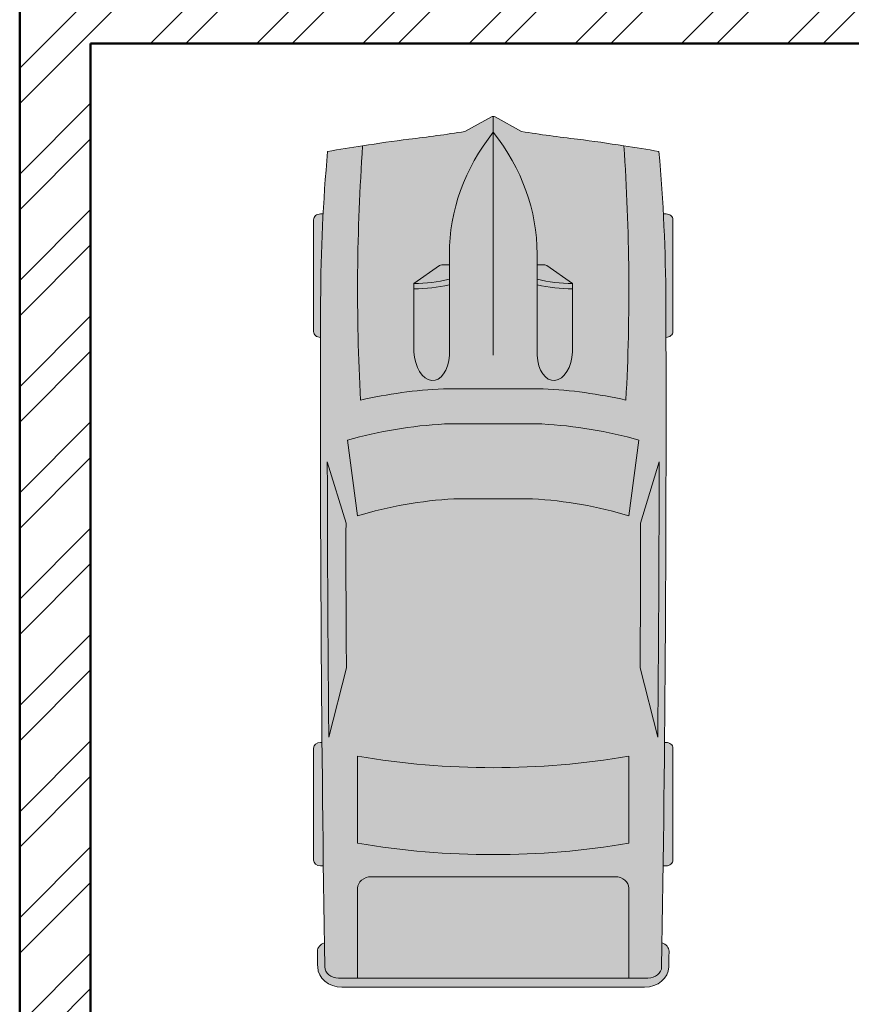
# Model space of a CAD drawing. Units: inches. Extents: x -31485 to -28799, y 18003 to 19130.
# Tile 1 of 15: x -31210 to -31104, y 18273 to 18398. Entities that reach past the tile are written whole.
import ezdxf

# ---------------------------------------------------------------- set-up
doc = ezdxf.new("R2010")
doc.units = ezdxf.units.IN
for name, color, linetype, lineweight in [('A-EQPM', 8, 'Continuous', 18), ('A-WALL', 7, 'Continuous', 50), ('A-WALL-PATT', 8, 'Continuous', 13)]:
    doc.layers.add(name, color=color, linetype=linetype, lineweight=lineweight)

# ---------------------------------------------------------------- blocks, each defined once
blk = doc.blocks.new('*U75')
for p, q in [((1182.463644577746, 987.7673041878503), (567.7039087844591, 987.7673041878503)), ((3472.124202183229, 987.7673041878503), (4086.88393797651, 987.767304187848)), ((536.0433148737552, 950.1792138851854), (536.0433148737552, 935.5404748014407)), ((1214.124238488447, 949.7089586534819), (1214.124238488447, 950.1792138851854)), ((3440.463608272525, 941.6679440245914), (3440.463608272525, 950.1792138851854)), ((4118.544531887212, 950.1792138851804), (4118.544531887212, 934.0601128753084)), ((2234.827175480885, 809.5287016048088), (1898.878785383111, 912.4126225124705)), ((3411.559256322833, 904.3494681924599), (3029.921878250559, 807.1504809911063)), ((4736.411271353851, -850.8646766016326), (4736.411271353883, 850.864676601626)), ((4785.334832293326, -832.0706314503777), (4785.334832293357, 832.0706314502926)), ((1778.76917512805, 801.0177247054045), (2194.716249451875, 745.5217224176465)), ((3515.941238262737, 745.5217224176508), (3994.062813016633, 745.5217224176508)), ((4736.411271353883, 745.5217224176529), (4242.012185201922, 745.5217224176529)), ((4178.690997380514, 670.345541812321), (4178.690997380509, -670.3455418123318)), ((819.5542361210883, 295.2827619512633), (917.6699264680983, 436.1082195367583)), ((917.6699264680983, 436.1082195367583), (1293.848362214069, 436.1082195367583)), ((815.9220749762081, 241.4481679439487), (815.9220749762081, 283.3039660446585)), ((1496.485716216861, -273.6820371142997), (1496.485716216861, 273.6820371142868)), ((756.2288711996046, 241.4481679439487), (1312.764151599097, 241.4481679439487)), ((1690.372337881975, -267.4332505757059), (1690.372337881975, 267.4332505756928)), ((4736.411271353883, -267.4332505757059), (4736.411271353883, 267.4332505756928)), ((2101.521373270556, 215.7994139342878), (2101.521373270556, -215.7994139342835)), ((82.96813941916749, 155.6585683733955), (2.596917328392246, 10.3141998552517)), ((-1.1252e-12, -6.4972e-12), (1312.764151599097, -6.4972e-12)), ((2.596917328392246, -10.31419985525964), (82.96813941916749, -155.6585683734063)), ((756.2288711996046, -241.4481679439617), (1312.764151599097, -241.4481679439617)), ((815.9220749762081, -241.4481679439617), (815.9220749762081, -283.3039660446715)), ((819.5542361210883, -295.2827619512763), (917.6699264680983, -436.1082195367712)), ((917.6699264680983, -436.1082195367712), (1293.848362214069, -436.1082195367712)), ((2194.716249451869, -745.5217224176688), (1778.769175128041, -801.0177247054262)), ((3994.062813016633, -745.5217224176616), (3515.941238262737, -745.5217224176638)), ((4242.012185201917, -745.5217224176638), (4736.411271353857, -745.5217224176594)), ((2234.827175480882, -809.5287016048153), (1898.878785383109, -912.4126225124726)), ((3411.559256322828, -904.349468192473), (3029.921878250557, -807.150480991115)), ((536.0433148737552, -950.1792138851984), (536.0433148737552, -935.5404748014537)), ((1214.124238488447, -949.7089586534948), (1214.124238488447, -950.1792138851984)), ((3440.463608272523, -941.6679440246044), (3440.463608272523, -950.1792138851984)), ((4118.544531887212, -950.1792138851933), (4118.544531887212, -934.0601128753214)), ((1182.463644577746, -987.7673041878633), (567.7039087844591, -987.7673041878633)), ((3472.124202183229, -987.7673041878633), (4086.883937976504, -987.767304187861))]:
    blk.add_line(p, q)
for centre, major_axis, ratio, start_param, end_param in [((567.7039087844591, 950.1792138851861), (5.296e-13, -37.5880903026662), 0.842303869543976, 3.141592653589776, 4.712388980384677), ((1182.463644577746, 950.1792138851861), (5.601e-13, 37.58809030266621), 0.8423038695439758, -1.570796326794884, 1.73e-14), ((3472.124202183229, 950.1792138851861), (5.988e-12, -37.5880903026662), 0.8423038695439762, 3.141592653589603, 4.712388980384554), ((4086.88393797651, 950.179213885181), (1.4197e-12, 37.5880903026662), 0.842303869543976, -1.570796326794865, 4.44e-14), ((1046.255263051279, -12467.92283887244), (3.2861e-12, 13417.14359589015), 0.8423038695439741, 0.0028100083536837, 0.0755983031096952), ((1637.842620806017, -268112.68896731), (4.8454159e-09, 269062.8681811952), 0.842303869543847, -0.0133969486112073, 0.0027970409639888), ((4587.952203166941, 910.2894362332722), (1.8792e-12, 56.38213545399769), 0.8423038695439691, -0.0130174256259048, 1.249894140392862), ((1637.84262086767, -268131.4830124673), (3.42859201765e-05, 269120.9512111412), 0.8423038681351471, -0.0133969484821159, -0.0130174254969711), ((4673.090083532475, 850.8646766015395), (7.5e-15, -75.17618060533067), 0.8423038695439952, 1.570796326796048, 3.128195704978389), ((4673.090083532448, 832.070631450172), (2.1733e-12, -133.2592106239272), 0.8423038695439737, 1.570796326795794, 3.128195704978164), ((6757.162543998887, -699.1204428451242), (4.9938223e-09, 7958.017136535005), 0.8423038695435286, 1.367075990158062, 1.391760499156098), ((1637.842620802809, -268112.6889680619), (4.87113144e-08, -269025.2800916445), 0.8423038695482963, 3.133765086725325, 3.140440689641252), ((3436.395912346701, 136.8410185571553), (5.76965e-11, 2077.023647078763), 0.8423038695439563, 1.245306111696802, 1.507880129813836), ((2433.035484508693, -93125.37499596032), (4.952654e-09, -93935.19844392464), 0.8423038695446962, 3.134048706297306, 3.14409775411291), ((6583.045501169266, -699.1204428451198), (3.826807e-09, -7754.693443154298), 0.8423038695443791, 4.528606069860317, 4.561837674556238), ((951.8333444315502, -15086.63944974413), (1.5767e-12, -15832.53653317094), 0.8423038695439826, 3.09604606856106, 3.200911180495224), ((3413.769624379244, 136.8410185571329), (1.08602e-11, -2280.347340451234), 0.84230386954398, 4.44948196380473, 4.652344057257214), ((3799.722190048092, 71.1058404433382), (2.17448e-11, -2021.323467232052), 0.842303869543983, 4.372215489277867, 4.640744122441986), ((433.884764992104, -3.6096e-12), (1.7438e-12, 3734.255266801694), 0.8423038695439766, 4.511394369635731, 4.913383591133647), ((912.0063397460013, -3.6096e-12), (1.7438e-12, 3734.255266801694), 0.8423038695439766, 4.511394369635731, 4.913383591133647), ((4242.012185201922, 670.3455418123216), (3.5405e-12, 75.17618060533239), 0.842303869543976, 5.55e-14, 1.57079632679492), ((-5194.164488957196, 1330.879982200552), (1.0466145e-09, -6374.389491984369), 0.8423038695441164, 1.385369446298923, 1.434372047871027), ((331.12799165183, 432.0470009052715), (3.125e-11, 696.3661584994836), 0.8423038695439277, 4.435146050259648, 4.718221029521873), ((360.7019022476185, 432.0470009052715), (3.125e-11, 696.3661584994836), 0.8423038695439277, 4.435146050259648, 4.718221029521873), ((1290.073045555822, 338.7781937403542), (161.0379696969085, -9.057857958340485), 0.6038335755719145, -1.39555193967809, 1.581314658479915), ((831.7523719315589, 283.3039660446593), (3.3347e-12, 18.79404515133458), 0.8423038695439091, 0.8797135699495516, 1.570796326795045), ((756.2288711996046, -1185.240851913765), (1.2998e-12, 1426.689019857713), 0.842303869543976, 7e-16, 0.5903187773915901), ((15.83029695535095, -3.6096e-12), (1.9e-15, -18.79404515133476), 0.842303869543842, 4.131459131953847, 5.293318828815531), ((756.2288711996046, 1185.240851913753), (1.01699e-11, 1426.689019857713), 0.8423038695439736, 2.55127387619821, 3.141592653589801), ((-5194.164488957196, -1330.879982200562), (1.0234792e-09, 6374.389491984348), 0.8423038695441192, -1.43437204787103, -1.385369446298926), ((3799.722190048497, -71.10584044329416), (1.038796e-10, -2021.323467232635), 0.8423038695439419, -1.499151468852248, -1.230622835688196), ((331.12799165183, -432.0470009052816), (3.1922e-11, -696.3661584994801), 0.842303869543932, 1.564964277657711, 1.848039256919935), ((360.7019022476185, -432.0470009052816), (3.1922e-11, -696.3661584994801), 0.842303869543932, 1.564964277657711, 1.848039256919935), ((3436.395912346742, -136.8410185572101), (8.13766e-11, -2077.023647078826), 0.8423038695439492, -1.50788012981387, -1.245306111696839), ((831.7523719315589, -283.3039660446737), (3.3028e-12, -18.79404515133458), 0.8423038695439093, 4.712388980384541, 5.403471737230034), ((3413.769624379237, -136.841018557156), (1.090899e-10, -2280.347340451348), 0.8423038695439354, -1.510751403667474, -1.307889310215002), ((6583.045501169163, 699.1204428449458), (2.756795e-10, 7754.693443157768), 0.8423038695439974, 1.721347632622872, 1.754579237318777), ((4242.012185201917, -670.3455418123318), (2.579e-13, -75.17618060533128), 0.8423038695439885, 4.712388980384686, 6.283185307179581), ((6757.162543998887, 699.1204428451076), (2.2231118e-09, 7958.017136528592), 0.8423038695441819, 1.749832154434603, 1.774516663432659), ((951.8333444315729, 15086.63944974408), (2.97009e-11, -15832.5365331709), 0.8423038695439528, -0.0593185269054384, 0.0455465850287298), ((2433.03548450906, 93125.37499596029), (4.1600574e-09, -93935.19844392457), 0.8423038695447548, -0.0025051005232382, 0.007543947292366), ((4673.090083532448, -850.8646766015358), (2.354e-13, 75.17618060532999), 0.8423038695439732, 3.154989602201626, 4.71238898038339), ((4673.090083532349, -832.0706314501077), (6.1679e-12, -133.2592106240062), 0.8423038695439807, 0.0133969486110846, 1.570796326792831), ((1046.255263051284, 12467.92283887242), (3.49903e-10, -13417.14359589015), 0.8423038695440652, -0.0755983031097181, -0.0028100083537155), ((1637.842620803916, 268112.6889680615), (4.0766478e-08, -269025.280091644), 0.8423038695397146, 0.0011519639481523, 0.0078275668641468), ((567.7039087844591, -950.1792138851977), (5.601e-13, 37.58809030266621), 0.8423038695439758, 1.570796326794908, 3.14159265358981), ((1637.842620801787, 268112.6889680619), (1.55395844e-08, 269062.868181947), 0.8423038695458147, 3.138795612625926, 3.154989602201039), ((1182.463644577746, -950.1792138851977), (5.296e-13, -37.5880903026662), 0.842303869543976, -1.69e-14, 1.570796326794884), ((3472.124202183229, -950.1792138851955), (3.96e-13, -37.58809030266733), 0.8423038695440105, -1.570796326794875, -1.27e-14), ((4086.883937976504, -950.1792138851933), (5.0003e-12, 37.58809030266732), 0.8423038695440109, 3.141592653589951, 4.712388980384771), ((4587.952203166856, -910.2894362333229), (5.777e-12, -56.38213545402103), 0.8423038695439803, -1.249894138785958, 0.0130174256254374), ((1637.842620726191, 268131.4830135791), (2.37878358395e-05, 269120.9512123862), 0.8423038705260315, 3.154610079306566, 3.154989602290631)]:
    blk.add_ellipse(centre, major_axis=major_axis, ratio=ratio, start_param=start_param, end_param=end_param)
at = {"extrusion": (0, 0, -1)}
blk.add_ellipse((1290.073045555822, -338.7781937403665), major_axis=(161.0379696969085, 9.057857958340424), ratio=0.6038335755719145, start_param=-1.39555193967809, end_param=1.581314658479915, dxfattribs=at)

msp = doc.modelspace()

# ---------------------------------------------------------------- hatches: boundary and pattern name
at = {"layer": 'A-EQPM'}
h = msp.add_hatch(color=256, dxfattribs=at)
h.dxf.hatch_style = 1
edge = h.paths.add_edge_path()
edge.add_ellipse((-24963.89229182593, 18347.74966155698), major_axis=(6207.481987576119, 3.1368e-12), ratio=0.84230386954367, start_angle=180.3838667787923, end_angle=180.5282714718174, ccw=False)
edge.add_line((-31171.17791802856, 18306.16184460638), (-31171.37427940205, 18306.16184460638))
edge.add_ellipse((-31171.37427940205, 18305.43141098043), major_axis=(-0.8671854094100128, 1.6795e-12), ratio=0.8423038695444475, start_angle=-89.99999999988903, end_angle=1.109639e-10)
edge.add_line((-31172.24146481146, 18305.43141098043), (-31172.24146481146, 18291.24844321379))
edge.add_ellipse((-31171.37427940205, 18291.24844321379), major_axis=(-0.8671854094100128, 3.5068e-12), ratio=0.8423038695402523, start_angle=2.317008e-10, end_angle=90.0000000002317)
edge.add_line((-31171.37427940205, 18290.51800958783), (-31171.00239966313, 18290.51800958783))
edge = h.paths.add_edge_path()
edge.add_ellipse((-31133.98755896982, 18287.66951830704), major_axis=(-1.734370818820025, 1.15572e-11), ratio=0.8423038695444475, start_angle=180.0000000003817, end_angle=270.0000000003818)
edge.add_line((-31133.98755896982, 18289.13038555896), (-31164.91830689776, 18289.13038555896))
edge.add_ellipse((-31164.91830689776, 18287.66951830704), major_axis=(1.734370818820025, 1.15576e-11), ratio=0.8423038695444475, start_angle=89.99999999961817, end_angle=179.9999999996181)
edge.add_line((-31166.65267771658, 18287.66951830704), (-31166.65267771658, 18276.26336091826))
edge.add_line((-31166.65267771658, 18276.26336091826), (-31132.253188151, 18276.26336091826))
edge.add_line((-31132.253188151, 18276.26336091826), (-31132.253188151, 18287.66951830704))
edge = h.paths.add_edge_path()
edge.add_ellipse((-31127.53158646552, 18305.43141098043), major_axis=(0.8671854094100124, 1.6795e-12), ratio=0.8423038695444477, start_angle=-1.109639e-10, end_angle=89.99999999988906)
edge.add_line((-31127.53158646552, 18306.16184460638), (-31127.72794783902, 18306.16184460638))
edge.add_ellipse((-37335.0135740243, 18347.74966155688), major_axis=(6207.481987558772, 4.152598e-10), ratio=0.8423038695472291, start_angle=-0.5282714718218244, end_angle=-0.38386677879640274, ccw=False)
edge.add_line((-31127.90346620446, 18290.51800958783), (-31127.53158646552, 18290.51800958783))
edge.add_ellipse((-31127.53158646552, 18291.24844321379), major_axis=(0.8671854094100124, 3.5068e-12), ratio=0.8423038695402528, start_angle=269.9999999997683, end_angle=359.9999999997682)
edge.add_line((-31126.66440105611, 18291.24844321379), (-31126.66440105611, 18305.43141098043))
edge = h.paths.add_edge_path()
edge.add_ellipse((-31497.51301000847, 18363.5764096146), major_axis=(365.2684817172168, 5.54988e-11), ratio=0.8423038695419378, start_angle=-2.198540565964143, end_angle=2.863714607828726)
edge.add_ellipse((-31165.58216542667, 18233.66012548605), major_axis=(-178.9065886093012, 1.2581094e-09), ratio=0.8423038695391548, start_angle=257.5553727069574, end_angle=259.7904610032577)
edge.add_ellipse((-31118.74853446752, 18505.36918505117), major_axis=(147.0619421407358, 1.9919546e-09), ratio=0.8423038695542743, start_angle=257.4450673550873, end_angle=260.74343399202326, ccw=False)
edge.add_line((-31145.86177312077, 18383.62178096662), (-31149.21497661432, 18385.47600528534))
edge.add_ellipse((-31149.45293293379, 18385.17070130109), major_axis=(-0.4335927046986816, 0), ratio=0.842303869552539, start_angle=232.0668695399768, end_angle=270)
edge.add_line((-31149.45293293379, 18385.53591811407), (-31149.45293293379, 18383.52118674771))
edge.add_ellipse((-31176.79732753163, 18368.08915138563), major_axis=(-32.91478475822442, 2.78257e-11), ratio=0.8423038695443898, start_angle=180.0000000000485, end_angle=209.438569598032, ccw=False)
edge.add_line((-31143.8825427734, 18368.08915138563), (-31143.8825427734, 18366.71198444421))
edge.add_line((-31143.8825427734, 18366.71198444421), (-31142.76081172944, 18366.71198444421))
edge.add_line((-31142.76081172944, 18366.71198444421), (-31139.39158951728, 18364.36458526691))
edge.add_line((-31139.39158951728, 18364.36458526691), (-31139.39158951728, 18355.68586687004))
edge.add_ellipse((-31141.63706614534, 18355.77296625432), major_axis=(0.2089715704820894, 3.715266632531377), ratio=0.6038335755718302, start_angle=106.3425919542722, end_angle=270.9979857249977, ccw=False)
edge.add_line((-31143.8825427734, 18355.24946543463), (-31143.8825427734, 18368.08915138563))
edge.add_ellipse((-31176.79732753163, 18368.08915138563), major_axis=(-32.91478475822442, 2.78257e-11), ratio=0.8423038695443898, start_angle=180.0000000000484, end_angle=209.4385695980319)
edge.add_ellipse((-31122.10853833595, 18368.08915138563), major_axis=(32.91478475822442, 2.78184e-11), ratio=0.8423038695443903, start_angle=150.561430401968, end_angle=179.9999999999515)
edge.add_line((-31155.02332309417, 18368.08915138563), (-31155.02332309417, 18355.24946543463))
edge.add_ellipse((-31157.26879972223, 18355.77296625432), major_axis=(-0.2089715704820894, 3.715266632531377), ratio=0.6038335755718302, start_angle=89.0020142750023, end_angle=253.6574080457279, ccw=False)
edge.add_line((-31159.51427635029, 18355.68586687004), (-31159.51427635029, 18364.36458526691))
edge.add_line((-31159.51427635029, 18364.36458526691), (-31156.14505413814, 18366.71198444421))
edge.add_line((-31156.14505413814, 18366.71198444421), (-31155.02332309417, 18366.71198444421))
edge.add_line((-31155.02332309417, 18366.71198444421), (-31155.02332309417, 18368.08915138563))
edge.add_ellipse((-31122.10853833595, 18368.08915138563), major_axis=(32.91478475822442, 2.78184e-11), ratio=0.8423038695443903, start_angle=150.5614304019681, end_angle=179.9999999999516, ccw=False)
edge.add_line((-31149.45293293379, 18383.52118674771), (-31149.45293293379, 18385.53591811407))
edge.add_ellipse((-31149.45293293379, 18385.17070130109), major_axis=(-0.4335927046986816, 0), ratio=0.842303869552539, start_angle=270, end_angle=307.9331304600232)
edge.add_line((-31149.69088925326, 18385.47600528534), (-31153.0440927468, 18383.62178096662))
edge.add_ellipse((-31180.15733140006, 18505.36918505117), major_axis=(-147.0619421372835, 4.9907306e-09), ratio=0.8423038695736066, start_angle=99.2565660091451, end_angle=102.55493264608151, ccw=False)
edge.add_ellipse((-31133.32370044092, 18233.66012548605), major_axis=(178.9065886092977, 1.2789651e-09), ratio=0.8423038695391513, start_angle=100.209538996733, end_angle=102.4446272930335)
edge.add_ellipse((-30801.39285585912, 18363.5764096146), major_axis=(365.2684817172171, 7.18011e-11), ratio=0.8423038695434502, start_angle=177.1362853921513, end_angle=182.1985405659441)
edge.add_ellipse((-31152.60995777187, 18306.77769481758), major_axis=(52.60932189168197, 7.16232e-11), ratio=0.8423038695431074, start_angle=94.08241069107589, end_angle=107.71995322267611, ccw=False)
edge.add_line((-31155.76698260995, 18351.01087126963), (-31143.13888325764, 18351.01087126963))
edge.add_ellipse((-31146.29590809571, 18306.77769481758), major_axis=(-52.6093218916263, 2.96862e-11), ratio=0.842303869543985, start_angle=252.2800467772827, end_angle=265.9175893088832, ccw=False)
h = msp.add_hatch(color=256, dxfattribs=at)
h.dxf.hatch_style = 1
edge = h.paths.add_edge_path()
edge.add_ellipse((-37335.0135740243, 18347.74966155688), major_axis=(6207.481987558772, 4.152598e-10), ratio=0.8423038695472291, start_angle=-0.3838667787963561, end_angle=0.0902290885904628)
edge.add_ellipse((-37335.0135740243, 18347.74966155688), major_axis=(6207.481987558772, 4.152598e-10), ratio=0.8423038695472291, start_angle=0.0902290885904628, end_angle=0.1349865768543979)
edge.add_ellipse((-31437.09725549581, 18361.39802519826), major_axis=(309.5435567121417, 3.12922e-11), ratio=0.8423038695440732, start_angle=0.1356123904321818, end_angle=2.179950313639523)
edge.add_ellipse((-31437.09725549581, 18361.39802519826), major_axis=(309.5435567121417, 3.12922e-11), ratio=0.8423038695440732, start_angle=2.179950313639523, end_angle=3.650427585692763)
edge.add_ellipse((-31165.58216542667, 18229.64311483572), major_axis=(183.5974185536168, 2.07254122e-08), ratio=0.8423038696260594, start_angle=76.2194710040335, end_angle=77.87403444124779)
edge.add_ellipse((-31497.51301000847, 18363.5764096146), major_axis=(365.2684817172168, 5.54988e-11), ratio=0.8423038695419378, start_angle=-2.1985405659640946, end_angle=2.8637146078286833, ccw=False)
edge.add_ellipse((-31146.29590809571, 18306.77769481758), major_axis=(-52.6093218916263, 2.96862e-11), ratio=0.842303869543985, start_angle=252.2800467772827, end_angle=265.9175893088831)
edge.add_line((-31143.13888325764, 18351.01087126963), (-31155.76698260995, 18351.01087126963))
edge.add_ellipse((-31152.60995777187, 18306.77769481758), major_axis=(52.60932189168197, 7.16232e-11), ratio=0.8423038695431074, start_angle=94.08241069107586, end_angle=107.719953222676)
edge.add_ellipse((-30801.39285585912, 18363.5764096146), major_axis=(365.2684817172171, 7.18011e-11), ratio=0.8423038695434502, start_angle=177.1362853921513, end_angle=182.1985405659441, ccw=False)
edge.add_ellipse((-31133.32370044092, 18229.64311483572), major_axis=(-183.5974185535601, 2.07797544e-08), ratio=0.8423038696263095, start_angle=-77.87403444123211, end_angle=-76.21947100401783)
edge.add_ellipse((-30861.80861037177, 18361.39802519826), major_axis=(-309.5435567121417, 3.20483e-11), ratio=0.8423038695440663, start_angle=-3.650427585692615, end_angle=-2.179950313639383)
edge.add_ellipse((-30861.80861037177, 18361.39802519826), major_axis=(-309.5435567121417, 3.20483e-11), ratio=0.8423038695440663, start_angle=-2.179950313639383, end_angle=-0.1356123904320413)
edge.add_ellipse((-24963.89229182593, 18347.74966155698), major_axis=(6207.481987576119, 3.1368e-12), ratio=0.84230386954367, start_angle=179.8650134231429, end_angle=179.9097709114068)
edge.add_ellipse((-24963.89229182593, 18347.74966155698), major_axis=(6207.481987576119, 3.1368e-12), ratio=0.84230386954367, start_angle=179.9097709114068, end_angle=180.3838667787923)
edge.add_ellipse((-24963.89229182593, 18347.74966155698), major_axis=(6207.481987576119, 3.1368e-12), ratio=0.84230386954367, start_angle=180.3838667787923, end_angle=180.5282714718173)
edge.add_ellipse((-24963.89229182593, 18347.74966155698), major_axis=(6207.481987576119, 3.1368e-12), ratio=0.84230386954367, start_angle=180.5282714718173, end_angle=180.6465540970609)
edge.add_ellipse((-31169.08301860692, 18277.72422817018), major_axis=(1.734370818820398, 6.2835e-12), ratio=0.8423038695442665, start_angle=180.6465540968934, end_angle=269.9999999996497)
edge.add_line((-31169.08301860692, 18276.26336091826), (-31166.65267771658, 18276.26336091826))
edge.add_line((-31166.65267771658, 18276.26336091826), (-31166.65267771658, 18287.86198447103))
edge.add_ellipse((-31164.91830689776, 18287.66951830704), major_axis=(1.734370818820025, 1.15576e-11), ratio=0.8423038695444475, start_angle=89.99999999961818, end_angle=179.9999999996182, ccw=False)
edge.add_line((-31164.91830689776, 18289.13038555896), (-31133.75905929062, 18289.13038555896))
edge.add_ellipse((-31133.98755896982, 18287.66951830704), major_axis=(-1.734370818820025, 1.15572e-11), ratio=0.8423038695444475, start_angle=180.0000000003818, end_angle=270.00000000038176, ccw=False)
edge.add_line((-31132.253188151, 18287.66951830704), (-31132.253188151, 18276.26336091826))
edge.add_line((-31132.253188151, 18276.26336091826), (-31129.82284726066, 18276.26336091826))
edge.add_ellipse((-31129.82284726066, 18277.72422817017), major_axis=(-1.734370818820364, 1.2413e-12), ratio=0.8423038695421853, start_angle=90.00000000018369, end_angle=179.3534459030602)
edge.add_ellipse((-37335.0135740243, 18347.74966155688), major_axis=(6207.481987558772, 4.152598e-10), ratio=0.8423038695472291, start_angle=-0.6465540970657812, end_angle=-0.6186431963230548)
edge.add_ellipse((-37335.0135740243, 18347.74966155688), major_axis=(6207.481987558772, 4.152598e-10), ratio=0.8423038695472291, start_angle=-0.6186431963230548, end_angle=-0.5282714718217923)
edge.add_ellipse((-37335.0135740243, 18347.74966155688), major_axis=(6207.481987558772, 4.152598e-10), ratio=0.8423038695472291, start_angle=-0.5282714718217923, end_angle=-0.3838667787963561)
edge = h.paths.add_edge_path(flags=16)
edge.add_ellipse((-29000.98074953765, 18329.40396632424), major_axis=(2167.155417170915, 1.2045892e-09), ratio=0.8423038695205244, start_angle=179.8791026309351, end_angle=180.3640763488582)
edge.add_line((-31168.07449935754, 18315.63334995188), (-31170.31695282702, 18306.82868966495))
edge.add_ellipse((-24963.89229182594, 18347.74966155692), major_axis=(6206.614802166701, 5.2511138e-09), ratio=0.842303869515611, start_angle=180.0555943134506, end_angle=180.3777641938611, ccw=False)
edge.add_line((-31170.5029758392, 18341.72736163617), (-31168.12936668919, 18333.97678053823))
edge = h.paths.add_edge_path(flags=16)
edge.add_ellipse((-31151.09339795501, 18297.87347991926), major_axis=(46.63344704056234, 1.445442e-10), ratio=0.842303869541784, start_angle=94.8700695969603, end_angle=112.7919148774121)
edge.add_line((-31166.65267771658, 18334.9021696583), (-31167.93301207454, 18344.49838034726))
edge.add_ellipse((-31152.60995777187, 18306.25568939947), major_axis=(47.91849192778146, 1.460375e-10), ratio=0.8423038695419556, start_angle=94.27742096287608, end_angle=111.8349537965307, ccw=False)
edge.add_line((-31155.62281842206, 18346.5377616215), (-31143.28304744552, 18346.5377616215))
edge.add_ellipse((-31146.29590809571, 18306.25568939947), major_axis=(-47.91849192778267, 1.361529e-10), ratio=0.8423038695419347, start_angle=248.1650462034528, end_angle=265.72257903710704, ccw=False)
edge.add_line((-31130.97285379305, 18344.49838034726), (-31132.253188151, 18334.9021696583))
edge.add_ellipse((-31147.81246791256, 18297.87347991927), major_axis=(-46.63344704055716, 1.546607e-10), ratio=0.8423038695417213, start_angle=247.208085122601, end_angle=265.1299304030565)
edge.add_line((-31144.47427874796, 18337.05224528612), (-31154.43158711963, 18337.05224528612))
edge = h.paths.add_edge_path(flags=16)
edge.add_ellipse((-31149.45293293379, 18375.52587146003), major_axis=(-86.15206721880882, 2.44e-14), ratio=0.8423038695434939, start_angle=76.40186530976904, end_angle=103.5981346902309)
edge.add_line((-31132.253188151, 18304.42051912437), (-31132.253188151, 18293.38989612087))
edge.add_ellipse((-31149.45293293379, 18364.49524845652), major_axis=(-86.15206721880666, 5.3e-15), ratio=0.8423038695434728, start_angle=76.40186530976843, end_angle=103.59813469023157, ccw=False)
edge.add_line((-31166.65267771658, 18293.38989612087), (-31166.65267771658, 18304.42051912437))
edge = h.paths.add_edge_path(flags=16)
edge.add_ellipse((-33297.92511632993, 18329.40396632425), major_axis=(-2167.155417170915, 1.2310555e-09), ratio=0.8423038695201377, start_angle=179.6359236511422, end_angle=180.1208973690652)
edge.add_line((-31130.77649917839, 18333.97678053823), (-31128.40289002838, 18341.72736163617))
edge.add_ellipse((-37335.01357404164, 18347.74966155695), major_axis=(-6206.614802166709, 5.3834157e-09), ratio=0.8423038695157945, start_angle=179.6222358061399, end_angle=179.9444056865504, ccw=False)
edge.add_line((-31128.58891304056, 18306.82868966495), (-31130.83136651004, 18315.63334995188))
h = msp.add_hatch(color=256, dxfattribs=at)
h.dxf.hatch_style = 1
edge = h.paths.add_edge_path()
edge.add_ellipse((-31127.53158646552, 18305.43141098043), major_axis=(0.8671854094100124, 1.6795e-12), ratio=0.8423038695444477, start_angle=-1.109639e-10, end_angle=89.99999999988906)
edge.add_line((-31127.53158646552, 18306.16184460638), (-31127.72794783902, 18306.16184460638))
edge.add_ellipse((-37335.0135740243, 18347.74966155688), major_axis=(6207.481987558772, 4.152598e-10), ratio=0.8423038695472291, start_angle=-0.5282714718218244, end_angle=-0.38386677879640274, ccw=False)
edge.add_line((-31127.90346620446, 18290.51800958783), (-31127.53158646552, 18290.51800958783))
edge.add_ellipse((-31127.53158646552, 18291.24844321379), major_axis=(0.8671854094100124, 3.5068e-12), ratio=0.8423038695402528, start_angle=269.9999999997683, end_angle=359.9999999997682)
edge.add_line((-31126.66440105611, 18291.24844321379), (-31126.66440105611, 18305.43141098043))
edge = h.paths.add_edge_path()
edge.add_line((-31171.17791802856, 18306.16184460638), (-31171.37427940205, 18306.16184460638))
edge.add_ellipse((-31171.37427940205, 18305.43141098043), major_axis=(-0.8671854094100128, 1.6795e-12), ratio=0.8423038695444475, start_angle=-89.99999999988903, end_angle=1.109639e-10)
edge.add_line((-31172.24146481146, 18305.43141098043), (-31172.24146481146, 18291.24844321379))
edge.add_ellipse((-31171.37427940205, 18291.24844321379), major_axis=(-0.8671854094100128, 3.5068e-12), ratio=0.8423038695402523, start_angle=2.317008e-10, end_angle=90.0000000002317)
edge.add_line((-31171.37427940205, 18290.51800958783), (-31171.00239966313, 18290.51800958783))
edge.add_ellipse((-24963.89229182593, 18347.74966155698), major_axis=(6207.481987576119, 3.1368e-12), ratio=0.84230386954367, start_angle=180.3838667787923, end_angle=180.5282714718174, ccw=False)
edge = h.paths.add_edge_path()
edge.add_ellipse((-31127.53158646552, 18372.43856353717), major_axis=(0.8671854094100124, 1.6795e-12), ratio=0.8423038695444477, start_angle=-1.109639e-10, end_angle=89.99999999988906)
edge.add_line((-31127.53158646552, 18373.16899716313), (-31127.86931314553, 18373.16899716313))
edge.add_ellipse((-31437.09725549581, 18361.39802519826), major_axis=(309.5435567121417, 3.12922e-11), ratio=0.8423038695440732, start_angle=0.1356123904321862, end_angle=2.1799503136394947, ccw=False)
edge.add_ellipse((-37335.0135740243, 18347.74966155688), major_axis=(6207.481987558772, 4.152598e-10), ratio=0.8423038695472291, start_angle=0.09022908859049039, end_angle=0.13498657685437365, ccw=False)
edge.add_line((-31127.5424356061, 18357.52516214458), (-31127.53158646552, 18357.52516214458))
edge.add_ellipse((-31127.53158646552, 18358.25559577054), major_axis=(-0.8671854094100128, 1.6795e-12), ratio=0.8423038695444475, start_angle=90.00000000011094, end_angle=180.0000000001109)
edge.add_line((-31126.66440105611, 18358.25559577054), (-31126.66440105611, 18372.43856353717))
edge = h.paths.add_edge_path()
edge.add_ellipse((-30861.80861037177, 18361.39802519826), major_axis=(-309.5435567121417, 3.20483e-11), ratio=0.8423038695440663, start_angle=-2.179950313639381, end_angle=-0.13561239043201567, ccw=False)
edge.add_line((-31171.03655272206, 18373.16899716313), (-31171.37427940205, 18373.16899716313))
edge.add_ellipse((-31171.37427940205, 18372.43856353717), major_axis=(-0.8671854094100128, 1.6795e-12), ratio=0.8423038695444475, start_angle=-89.99999999988903, end_angle=1.109639e-10)
edge.add_line((-31172.24146481146, 18372.43856353717), (-31172.24146481146, 18358.25559577054))
edge.add_ellipse((-31171.37427940205, 18358.25559577054), major_axis=(0.8671854094100124, 1.6795e-12), ratio=0.8423038695444477, start_angle=179.999999999889, end_angle=269.999999999889)
edge.add_line((-31171.37427940205, 18357.52516214458), (-31171.36343026148, 18357.52516214458))
edge.add_ellipse((-24963.89229182593, 18347.74966155698), major_axis=(6207.481987576119, 3.1368e-12), ratio=0.84230386954367, start_angle=179.865013423143, end_angle=179.9097709114068, ccw=False)
edge = h.paths.add_edge_path()
edge.add_ellipse((-31139.48528487433, 18377.21425494213), major_axis=(16.06568908904641, 9.1463e-11), ratio=0.8423038695487669, start_angle=251.332504507076, end_angle=270.3967098596572, ccw=False)
edge.add_line((-31143.8825427734, 18364.19880697911), (-31143.8825427734, 18355.24946543463))
edge.add_ellipse((-31141.63706614534, 18355.77296625432), major_axis=(0.2089715704820894, 3.715266632531377), ratio=0.6038335755718302, start_angle=106.3425919542721, end_angle=270.9979857249977)
edge.add_line((-31139.39158951728, 18355.68586687004), (-31139.39158951728, 18363.68229298866))
edge = h.paths.add_edge_path()
edge.add_ellipse((-31142.91689814715, 18366.34676763123), major_axis=(-0.4335927047225754, 4.1219e-11), ratio=0.8423038695061223, start_angle=225.5197891228621, end_angle=270.0000000054467)
edge.add_line((-31142.91689814715, 18366.71198444421), (-31143.8825427734, 18366.71198444421))
edge.add_line((-31143.8825427734, 18366.71198444421), (-31143.8825427734, 18364.88109925737))
edge.add_ellipse((-31139.48528487433, 18377.89654722039), major_axis=(-16.06568908915088, 3.60949e-11), ratio=0.8423038695435023, start_angle=71.33250450753091, end_angle=90.39670986011207)
edge.add_line((-31139.39158951728, 18364.36458526691), (-31142.64053834943, 18366.62818776489))
edge = h.paths.add_edge_path()
edge.add_line((-31155.02332309417, 18366.71198444421), (-31155.98896772044, 18366.71198444421))
edge.add_ellipse((-31155.98896772044, 18366.34676763123), major_axis=(0.4335927047225755, 4.12191e-11), ratio=0.8423038695061222, start_angle=89.99999999455322, end_angle=134.4802108771379)
edge.add_line((-31156.26532751815, 18366.62818776489), (-31159.51427635029, 18364.36458526691))
edge.add_ellipse((-31159.42058099325, 18377.89654722039), major_axis=(16.06568908915091, 3.60949e-11), ratio=0.8423038695435009, start_angle=269.6032901398879, end_angle=288.6674954924691)
edge.add_line((-31155.02332309417, 18364.88109925737), (-31155.02332309417, 18366.71198444421))
edge = h.paths.add_edge_path()
edge.add_ellipse((-31159.42058099325, 18377.21425494213), major_axis=(-16.06568908904639, 9.1463e-11), ratio=0.8423038695487673, start_angle=89.60329014034278, end_angle=108.66749549292399, ccw=False)
edge.add_line((-31159.51427635029, 18363.68229298866), (-31159.51427635029, 18355.68586687004))
edge.add_ellipse((-31157.26879972223, 18355.77296625432), major_axis=(-0.2089715704820894, 3.715266632531377), ratio=0.6038335755718302, start_angle=89.00201427500228, end_angle=253.6574080457278)
edge.add_line((-31155.02332309417, 18355.24946543463), (-31155.02332309417, 18364.19880697911))
h = msp.add_hatch(color=256, dxfattribs=at)
h.dxf.hatch_style = 1
edge = h.paths.add_edge_path()
edge.add_ellipse((-31139.48528487433, 18377.89654722039), major_axis=(-16.06568908915088, 3.60949e-11), ratio=0.8423038695435023, start_angle=71.33250450753093, end_angle=90.39670986011208, ccw=False)
edge.add_line((-31143.8825427734, 18364.88109925737), (-31143.8825427734, 18364.19880697911))
edge.add_ellipse((-31139.48528487433, 18377.21425494213), major_axis=(16.06568908904641, 9.1463e-11), ratio=0.8423038695487669, start_angle=251.332504507076, end_angle=270.3967098596572)
edge.add_line((-31139.39158951728, 18363.68229298866), (-31139.39158951728, 18364.36458526691))
edge = h.paths.add_edge_path()
edge.add_ellipse((-31159.42058099325, 18377.89654722039), major_axis=(16.06568908915091, 3.60949e-11), ratio=0.8423038695435009, start_angle=269.6032901398879, end_angle=288.667495492469, ccw=False)
edge.add_line((-31159.51427635029, 18364.36458526691), (-31159.51427635029, 18363.68229298866))
edge.add_ellipse((-31159.42058099325, 18377.21425494213), major_axis=(-16.06568908904639, 9.1463e-11), ratio=0.8423038695487673, start_angle=89.60329014034272, end_angle=108.667495492924)
edge.add_line((-31155.02332309417, 18364.19880697911), (-31155.02332309417, 18364.88109925737))
h = msp.add_hatch(color=256, dxfattribs=at)
h.dxf.hatch_style = 1
edge = h.paths.add_edge_path()
edge.add_ellipse((-31146.29590809571, 18306.25568939947), major_axis=(-47.91849192778267, 1.361529e-10), ratio=0.8423038695419347, start_angle=248.1650462034528, end_angle=265.722579037107)
edge.add_line((-31143.28304744552, 18346.5377616215), (-31155.62281842206, 18346.5377616215))
edge.add_ellipse((-31152.60995777187, 18306.25568939947), major_axis=(47.91849192778146, 1.460375e-10), ratio=0.8423038695419556, start_angle=94.277420962876, end_angle=111.8349537965306)
edge.add_line((-31167.93301207454, 18344.49838034726), (-31166.65267771658, 18334.9021696583))
edge.add_ellipse((-31151.09339795501, 18297.87347991926), major_axis=(46.63344704056234, 1.445442e-10), ratio=0.842303869541784, start_angle=94.8700695969602, end_angle=112.7919148774121, ccw=False)
edge.add_line((-31154.43158711963, 18337.05224528612), (-31144.47427874796, 18337.05224528612))
edge.add_ellipse((-31147.81246791256, 18297.87347991927), major_axis=(-46.63344704055716, 1.546607e-10), ratio=0.8423038695417213, start_angle=247.20808512260112, end_angle=265.1299304030565, ccw=False)
edge.add_line((-31132.253188151, 18334.9021696583), (-31130.97285379305, 18344.49838034726))
edge = h.paths.add_edge_path()
edge.add_ellipse((-29000.98074953765, 18329.40396632424), major_axis=(2167.155417170915, 1.2045892e-09), ratio=0.8423038695205244, start_angle=179.8791026309352, end_angle=180.3640763488582, ccw=False)
edge.add_line((-31168.12936668919, 18333.97678053823), (-31170.5029758392, 18341.72736163617))
edge.add_ellipse((-24963.89229182594, 18347.74966155692), major_axis=(6206.614802166701, 5.2511138e-09), ratio=0.842303869515611, start_angle=180.0555943134505, end_angle=180.377764193861)
edge.add_line((-31170.31695282702, 18306.82868966495), (-31168.07449935754, 18315.63334995188))
edge = h.paths.add_edge_path()
edge.add_ellipse((-37335.01357404164, 18347.74966155695), major_axis=(-6206.614802166709, 5.3834157e-09), ratio=0.8423038695157945, start_angle=179.6222358061398, end_angle=179.9444056865503)
edge.add_line((-31128.40289002838, 18341.72736163617), (-31130.77649917839, 18333.97678053823))
edge.add_ellipse((-33297.92511632993, 18329.40396632425), major_axis=(-2167.155417170915, 1.2310555e-09), ratio=0.8423038695201377, start_angle=179.6359236511423, end_angle=180.1208973690653, ccw=False)
edge.add_line((-31130.83136651004, 18315.63334995188), (-31128.58891304056, 18306.82868966495))
edge = h.paths.add_edge_path()
edge.add_ellipse((-31149.45293293379, 18375.52587146003), major_axis=(-86.15206721880882, 2.44e-14), ratio=0.8423038695434939, start_angle=76.40186530976911, end_angle=103.598134690231, ccw=False)
edge.add_line((-31166.65267771658, 18304.42051912437), (-31166.65267771658, 18293.38989612087))
edge.add_ellipse((-31149.45293293379, 18364.49524845652), major_axis=(-86.15206721880666, 5.3e-15), ratio=0.8423038695434728, start_angle=76.40186530976838, end_angle=103.5981346902316)
edge.add_line((-31132.253188151, 18293.38989612087), (-31132.253188151, 18304.42051912437))
edge = h.paths.add_edge_path()
edge.add_ellipse((-31130.25643996537, 18277.72422817018), major_axis=(3.074389845080431, 4.5193e-12), ratio=0.8423038695441155, start_angle=269.9999999999962, end_angle=359.3534459027799)
edge.add_ellipse((-37335.44716672914, 18347.74966155546), major_axis=(6208.82200659716, 5.2733622375e-06), ratio=0.8423038788855755, start_angle=-0.646554145712032, end_angle=-0.6282372648788858)
edge.add_ellipse((-31128.45187352682, 18279.68842286712), major_axis=(-1.30077811411332, 2.65586e-11), ratio=0.8423038695457158, start_angle=179.3717627849924, end_angle=248.4647566023133)
edge.add_ellipse((-37335.0135740243, 18347.74966155688), major_axis=(6207.481987558772, 4.152598e-10), ratio=0.8423038695472291, start_angle=-0.6465540970658026, end_angle=-0.6186431963230916, ccw=False)
edge.add_ellipse((-31129.82284726066, 18277.72422817017), major_axis=(-1.734370818820364, 1.2413e-12), ratio=0.8423038695421853, start_angle=90.00000000018372, end_angle=179.3534459030602, ccw=False)
edge.add_line((-31129.82284726066, 18276.26336091826), (-31169.08301860692, 18276.26336091826))
edge.add_ellipse((-31169.08301860692, 18277.72422817018), major_axis=(1.734370818820398, 6.2835e-12), ratio=0.8423038695442665, start_angle=180.6465540968934, end_angle=269.99999999964973, ccw=False)
edge.add_ellipse((-24963.89229182593, 18347.74966155698), major_axis=(6207.481987576119, 3.1368e-12), ratio=0.84230386954367, start_angle=180.5282714718174, end_angle=180.6465540970609, ccw=False)
edge.add_ellipse((-31170.45399234076, 18279.68842286712), major_axis=(1.300778114113422, 3.7711e-12), ratio=0.8423038695465029, start_angle=111.5352435038071, end_angle=180.6282372160113)
edge.add_ellipse((-24963.45869911279, 18347.74966155872), major_axis=(-6208.822006624284, 5.909233014e-06), ratio=0.842303880027109, start_angle=0.6282372707742053, end_angle=0.6465541516072572)
edge.add_ellipse((-31168.64942590221, 18277.72422817018), major_axis=(-3.074389845084005, 2.9376e-12), ratio=0.8423038695431365, start_angle=0.6465540971220629, end_angle=89.99999999989375)
edge.add_line((-31168.64942590221, 18275.13465770718), (-31130.25643996536, 18275.13465770718))
at = {"layer": 'A-WALL-PATT'}
h = msp.add_hatch(dxfattribs=at)
h.set_pattern_fill('ANSI32', color=256)
h.set_pattern_definition([(45, (-1687.357050595019, -0.3129728357926069), (-6.735192090801865, 6.735192090801866), []), (45, (-1682.866920595021, -0.3129728357926069), (-6.735192090801865, 6.735192090801866), [])])
h.paths.add_polyline_path([(-31156.52828769349, 18823.80296009311), (-31209.52828769349, 18823.80296009311), (-31209.52828769349, 18761.80296009311), (-31200.52828769349, 18761.80296009311), (-31200.52828769349, 18814.80296009311), (-31156.52828769349, 18814.80296009311)], flags=17)
h.paths.add_polyline_path([(-31022.5282876935, 18823.80296009311), (-31118.52828769349, 18823.80296009311), (-31118.52828769349, 18814.80296009311), (-31074.52828769349, 18814.80296009311), (-31074.52828769349, 18720.78574754094), (-31070.95696393926, 18720.78574754094), (-31068.52828769349, 18720.75952290947), (-31068.52828769349, 18814.80296009311), (-31022.5282876935, 18814.80296009311)], flags=17)
h.paths.add_polyline_path([(-30754.52828769349, 18823.80296009311), (-30850.5282876935, 18823.80296009311), (-30850.5282876935, 18814.80296009311), (-30806.5282876935, 18814.80296009311), (-30806.52828769349, 18723.10029278397), (-30800.5282876935, 18723.10029278397), (-30800.5282876935, 18814.80296009311), (-30754.52828769349, 18814.80296009311)], flags=17)
h.paths.add_polyline_path([(-30661.52828769349, 18823.80296009311), (-30716.52828769349, 18823.80296009311), (-30716.52828769349, 18814.80296009311), (-30670.52828769349, 18814.80296009311), (-30670.52828769349, 18761.80296009311), (-30661.52828769349, 18761.80296009311)], flags=17)
h.paths.add_polyline_path([(-30986.91891278487, 18670.80296009311), (-31068.52828769349, 18670.80296009311), (-31068.52828769349, 18684.75952290947), (-31074.52828769349, 18684.75952290947), (-31074.52828769349, 18670.80296009311), (-31200.52828769349, 18670.80296009311), (-31200.52828769349, 18723.80296009311), (-31209.52828769349, 18723.80296009311), (-31209.52828769349, 18641.80296009311), (-31200.52828769349, 18641.80296009311), (-31200.52828769349, 18664.80296009311), (-31104.52828769349, 18664.80296009311), (-31104.52828769349, 18628.92834044014), (-31098.52828769349, 18628.92834044014), (-31098.52828769348, 18664.8029600931), (-30986.91891278488, 18664.8029600931)], flags=17)
h.paths.add_polyline_path([(-30661.52828769349, 18723.80296009311), (-30670.52828769349, 18723.80296009311), (-30670.52828769349, 18670.80296009311), (-30800.5282876935, 18670.80296009311), (-30800.5282876935, 18687.10029278396), (-30806.52828769349, 18687.10029278396), (-30806.52828769349, 18670.80296009311), (-30885.59628027248, 18670.80296009311), (-30885.59628027248, 18667.80293426455), (-30885.59628027248, 18664.80296009311), (-30760.52828769349, 18664.80296009311), (-30760.52828769349, 18625.80296009311), (-30754.52828769349, 18625.80296009311), (-30754.52828769349, 18664.80296009311), (-30670.52828769349, 18664.80296009311), (-30670.52828769349, 18641.80296009311), (-30661.52828769349, 18641.80296009311)], flags=17)
h.paths.add_polyline_path([(-31200.52828769349, 18574.80296009311), (-31188.56436894977, 18574.80296009311), (-31188.56436894977, 18580.80296009311), (-31200.52828769349, 18580.80296009311), (-31200.52828769349, 18603.80296009311), (-31209.52828769349, 18603.80296009311), (-31209.52828769349, 18557.80296009311), (-31200.52828769349, 18557.80296009311)], flags=17)
h.paths.add_polyline_path([(-31098.52828769349, 18592.92834044014), (-31104.52828769349, 18592.92834044014), (-31104.52828769349, 18580.80296009311), (-31164.56436894977, 18580.80296009311), (-31164.56436894977, 18574.80296009311), (-31104.52828769349, 18574.80296009311), (-31104.52828769349, 18514.80296009311), (-31200.52828769349, 18514.80296009311), (-31200.52828769349, 18531.80296009311), (-31209.52828769349, 18531.80296009311), (-31209.52828769349, 18473.80296009311), (-31200.52828769349, 18473.80296009311), (-31200.52828769349, 18508.80296009311), (-31056.52828769349, 18508.80296009312), (-31056.52828769349, 18501.62307445529), (-31050.52828769349, 18501.62307445529), (-31050.52828769349, 18514.80296009311), (-31098.52828769349, 18514.80296009311)], flags=17)
h.paths.add_polyline_path([(-30661.52828769349, 18531.80296009311), (-30670.52828769349, 18531.80296009311), (-30670.52828769349, 18514.80296009311), (-30754.52828769349, 18514.80296009311), (-30754.52828769349, 18574.80296009311), (-30700.74522746605, 18574.80296009311), (-30700.74522746605, 18577.44024221289), (-30700.74522746605, 18580.8029600931), (-30754.52828769349, 18580.80296009311), (-30754.52828769349, 18589.80296009311), (-30760.52828769349, 18589.80296009311), (-30760.52828769349, 18514.80296009311), (-30820.52828769349, 18514.80296009311), (-30820.52828769348, 18499.26438911774), (-30814.52828769349, 18499.26438911774), (-30814.52828769349, 18508.80296009311), (-30670.52828769349, 18508.80296009311), (-30670.52828769349, 18473.80296009311), (-30661.52828769349, 18473.80296009311)], flags=17)
h.paths.add_polyline_path([(-30661.52828769349, 18435.80296009311), (-30670.52828769349, 18435.80296009311), (-30670.52828769349, 18400.80296009311), (-30814.52828769349, 18400.80296009311), (-30814.52828769349, 18413.15176302367), (-30820.52828769349, 18413.15176302367), (-30820.52828769349, 18400.80296009311), (-30932.52828769349, 18400.80296009311), (-30932.52828769349, 18664.80296009311), (-30921.59628027248, 18664.80296009311), (-30921.59628027248, 18670.80296009311), (-30932.5282876935, 18670.80296009311), (-30932.5282876935, 18814.80296009311), (-30888.5282876935, 18814.80296009311), (-30888.5282876935, 18823.80296009311), (-30984.5282876935, 18823.80296009311), (-30984.5282876935, 18814.80296009311), (-30938.5282876935, 18814.80296009311), (-30938.5282876935, 18670.80296009311), (-30950.91891278487, 18670.80296009311), (-30950.91891278488, 18664.80296009311), (-30938.5282876935, 18664.80296009311), (-30938.52828769349, 18400.80296009311), (-31050.52828769349, 18400.80296009311), (-31050.52828769349, 18411.18080736427), (-31056.52828769348, 18411.18080736427), (-31056.52828769348, 18400.80296009311), (-31200.52828769349, 18400.80296009311), (-31200.52828769349, 18435.80296009311), (-31209.52828769349, 18435.80296009311), (-31209.52828769349, 18179.80296009311), (-31200.52828769349, 18179.80296009311), (-31200.52828769349, 18394.80296009311), (-31001.52828769348, 18394.80296009311), (-31001.52828769348, 18179.80296009311), (-30954.52828769347, 18179.80296009311), (-30954.52828769347, 18188.80296009311), (-30995.52828769348, 18188.80296009311), (-30995.52828769348, 18394.80296009311), (-30875.52828769348, 18394.80296009311), (-30875.52828769348, 18188.80296009311), (-30916.52828769347, 18188.80296009311), (-30916.52828769347, 18179.80296009311), (-30869.52828769348, 18179.80296009311), (-30869.52828769348, 18394.80296009311), (-30670.52828769349, 18394.80296009311), (-30670.52828769349, 18179.80296009311), (-30661.52828769349, 18179.80296009311)])

# ---------------------------------------------------------------- linework, layer by layer
at = {"layer": 'A-WALL'}
for p, q in [((-31209.52828769349, 18179.80296009311), (-31209.52828769349, 18823.80296009311)), ((-31200.52828769349, 18394.80296009311), (-31001.52828769348, 18394.80296009311)), ((-31200.52828769349, 18179.80296009311), (-31200.52828769349, 18394.80296009311))]:
    msp.add_line(p, q, dxfattribs=at)

# ---------------------------------------------------------------- block references
at = {"layer": 'A-EQPM', "xscale": 0.0230707493364654, "yscale": 0.0230707493364654, "zscale": 0.0230707493364654, "rotation": 270}
msp.add_blockref('*U75', (-31149.45293293379, 18385.53591811407), dxfattribs=at)

doc.saveas('drawing.dxf')
